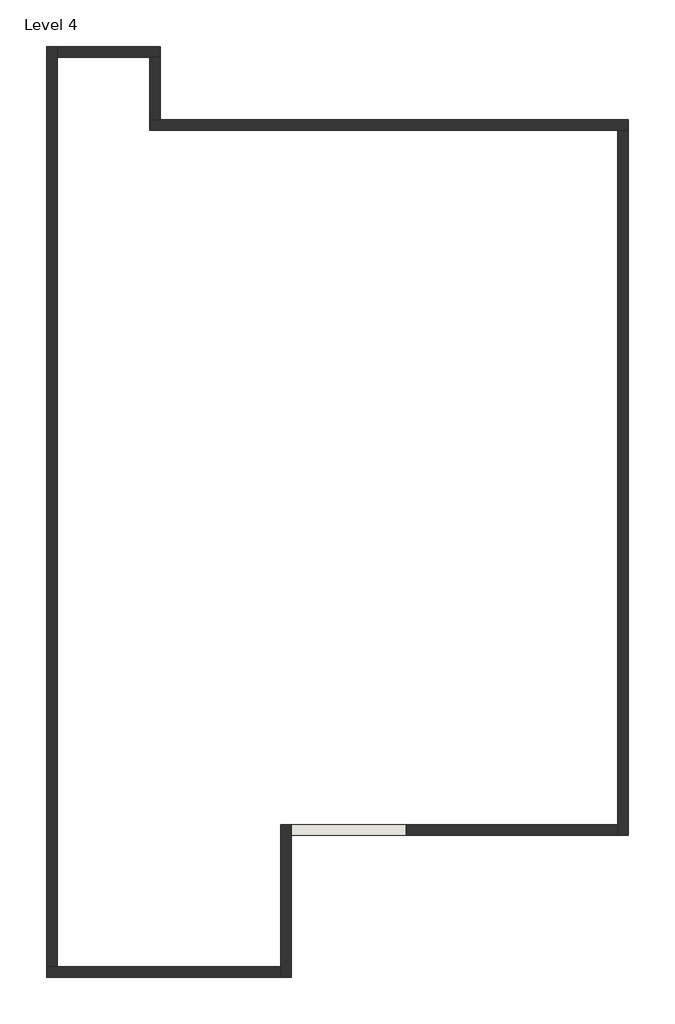
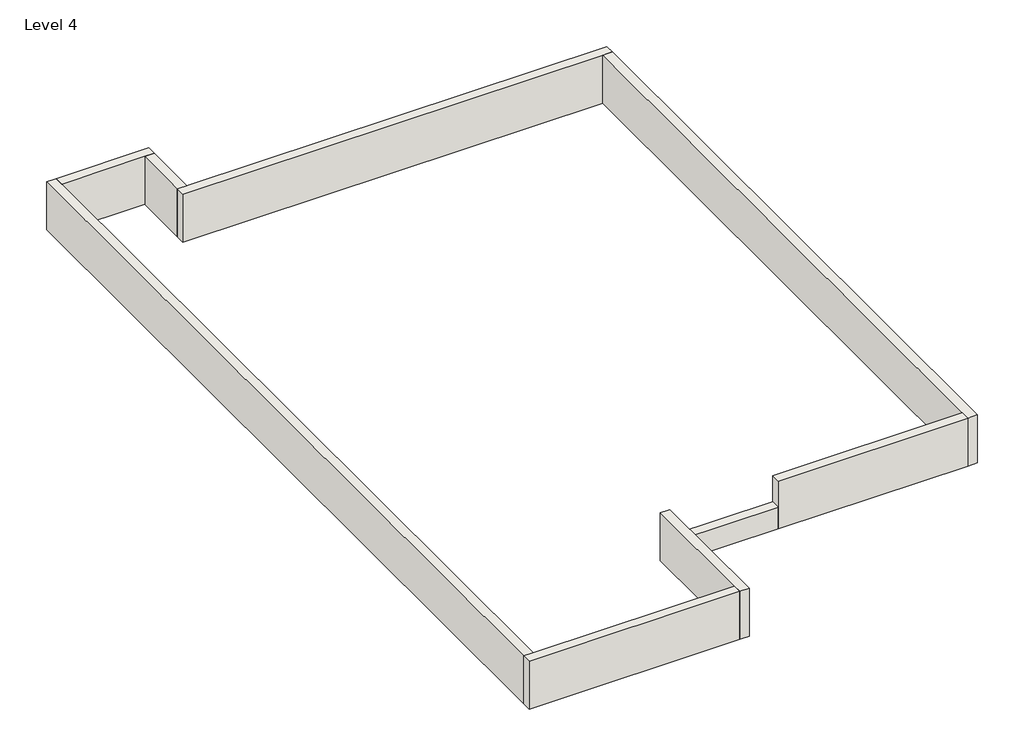
# One storey: 9 walls.
"""IFC4 building model written with IfcOpenShell, lengths in millimetres."""

from ifc_helpers import new_model, si_unit, frame, origin, place, context, project, spatial, polyline, outline, extrude, faceted_brep, element, save

model = new_model("IFC4")

# Units and contexts
model_context = context("Model", 3, world=origin())
ifc_project = project(units=[si_unit("LENGTHUNIT", "METRE", prefix="MILLI")], contexts=[model_context])

# Site, building, storey
site = spatial("IfcSite", under=ifc_project)
building = spatial("IfcBuilding", under=site)
storey = spatial("IfcBuildingStorey", under=building, Name="Level 4", Elevation=6858.0)

# Walls
placement = place(None, origin())
element("IfcWall", 1, ObjectType="9\" wall", at=placement, inside=storey, context=model_context, shape_type="Brep", body=[
    faceted_brep([(-5476.8909398, -2669.4648025, 6858.0), (-5476.8909398, -5745.6380415, 6858.0), (-5476.8909398, -5974.2380415, 6858.0), (-5476.8909398, -5974.2380415, 8077.2), (-5476.8909398, -5745.6380415, 8077.2), (-5476.8909398, -2669.4648025, 8077.2), (-5248.2909398, -2669.4648025, 6858.0), (-5248.2909398, -2669.4648025, 7414.0853363), (-5248.2909398, -2669.4648025, 8077.2), (-5248.2909398, -5974.2380415, 8077.2), (-5248.2909398, -5974.2380415, 6858.0), (-5248.2909398, -2898.0648025, 6858.0)], [[[0, 1, 2, 3, 4, 5]], [[6, 7, 8, 9, 10, 11]], [[2, 1, 0, 6, 11, 10]], [[5, 4, 3, 9, 8]], [[3, 2, 10, 9]], [[0, 5, 8, 7, 6]]]),
])
element("IfcWall", 2, ObjectType="9\" wall", at=placement, inside=storey, context=model_context, shape_type="Brep", body=[
    faceted_brep([(-5476.8909398, -5745.6380415, 6858.0), (-10315.5909398, -5745.6380415, 6858.0), (-10544.1909398, -5745.6380415, 6858.0), (-10544.1909398, -5745.6380415, 8077.2), (-10315.5909398, -5745.6380415, 8077.2), (-5476.8909398, -5745.6380415, 8077.2), (-5476.8909398, -5974.2380415, 6858.0), (-5476.8909398, -5974.2380415, 8077.2), (-10544.1909398, -5974.2380415, 8077.2), (-10544.1909398, -5974.2380415, 6858.0)], [[[0, 1, 2, 3, 4, 5]], [[6, 7, 8, 9]], [[2, 1, 0, 6, 9]], [[5, 4, 3, 8, 7]], [[0, 5, 7, 6]], [[3, 2, 9, 8]]]),
])
element("IfcWall", 3, ObjectType="9\" wall", at=placement, inside=storey, context=model_context, shape_type="Brep", body=[
    faceted_brep([(-10315.5909398, -5745.6380415, 6858.0), (-10315.5909398, 13923.3493277, 6858.0), (-10315.5909398, 14151.9493277, 6858.0), (-10315.5909398, 14151.9493277, 8077.2), (-10315.5909398, 13923.3493277, 8077.2), (-10315.5909398, -5745.6380415, 8077.2), (-10544.1909398, -5745.6380415, 6858.0), (-10544.1909398, -5745.6380415, 8077.2), (-10544.1909398, 14151.9493277, 8077.2), (-10544.1909398, 14151.9493277, 6858.0)], [[[0, 1, 2, 3, 4, 5]], [[6, 7, 8, 9]], [[2, 1, 0, 6, 9]], [[5, 4, 3, 8, 7]], [[0, 5, 7, 6]], [[3, 2, 9, 8]]]),
])
element("IfcWall", 4, ObjectType="9\" wall", at=placement, inside=storey, context=model_context, shape_type="Brep", body=[
    faceted_brep([(-8309.5689749, 12341.9351975, 6858.0), (1800.2090602, 12341.9351975, 6858.0), (2028.8090602, 12341.9351975, 6858.0), (2028.8090602, 12341.9351975, 8077.2), (1800.2090602, 12341.9351975, 8077.2), (-8309.5689749, 12341.9351975, 8077.2), (-8309.5689749, 12570.5351975, 6858.0), (-8309.5689749, 12570.5351975, 8077.2), (-8080.9689749, 12570.5351975, 8077.2), (2028.8090602, 12570.5351975, 8077.2), (2028.8090602, 12570.5351975, 6858.0), (-8080.9689749, 12570.5351975, 6858.0)], [[[0, 1, 2, 3, 4, 5]], [[6, 7, 8, 9, 10, 11]], [[2, 1, 0, 6, 11, 10]], [[5, 4, 3, 9, 8, 7]], [[3, 2, 10, 9]], [[0, 5, 7, 6]]]),
])
element("IfcWall", 5, ObjectType="9\" wall", at=placement, inside=storey, context=model_context, shape_type="Brep", body=[
    faceted_brep([(1800.2090602, 12341.9351975, 6858.0), (1800.2090602, -2669.4648025, 6858.0), (1800.2090602, -2783.7648025, 6858.0), (1800.2090602, -2898.0648025, 6858.0), (1800.2090602, -2898.0648025, 8077.2), (1800.2090602, -2669.4648025, 8077.2), (1800.2090602, 12341.9351975, 8077.2), (2028.8090602, 12341.9351975, 6858.0), (2028.8090602, 12341.9351975, 8077.2), (2028.8090602, -2898.0648025, 8077.2), (2028.8090602, -2898.0648025, 6858.0), (2028.8090602, -2783.7648025, 6858.0)], [[[0, 1, 2, 3, 4, 5, 6]], [[7, 8, 9, 10, 11]], [[3, 2, 1, 0, 7, 11, 10]], [[6, 5, 4, 9, 8]], [[0, 6, 8, 7]], [[4, 3, 10, 9]]]),
])
element("IfcWall", 6, ObjectType="9\" wall", at=placement, inside=storey, context=model_context, shape_type="Brep", body=[
    faceted_brep([(-10315.5909398, 13923.3493277, 6858.0), (-8309.5689749, 13923.3493277, 6858.0), (-8080.9689749, 13923.3493277, 6858.0), (-8080.9689749, 13923.3493277, 8077.2), (-8309.5689749, 13923.3493277, 8077.2), (-10315.5909398, 13923.3493277, 8077.2), (-10315.5909398, 14151.9493277, 6858.0), (-10315.5909398, 14151.9493277, 8077.2), (-8080.9689749, 14151.9493277, 8077.2), (-8080.9689749, 14151.9493277, 6858.0)], [[[0, 1, 2, 3, 4, 5]], [[6, 7, 8, 9]], [[2, 1, 0, 6, 9]], [[5, 4, 3, 8, 7]], [[3, 2, 9, 8]], [[0, 5, 7, 6]]]),
])
element("IfcWall", 7, ObjectType="9\" wall", at=placement, inside=storey, context=model_context, shape_type="SweptSolid", body=[
    extrude(outline(polyline([(-8309.5689749, 12570.5351975), (-8309.5689749, 13923.3493277), (-8080.9689749, 13923.3493277), (-8080.9689749, 12570.5351975), (-8309.5689749, 12570.5351975)])), frame((0.0, 0.0, 6858.0), z_axis=(0.0, 0.0, 1.0), x_axis=(1.0, 0.0, 0.0)), (0.0, 0.0, 1.0), 1219.2),
])
element("IfcWall", 8, ObjectType="9\" wall", at=placement, inside=storey, context=model_context, shape_type="Brep", body=[
    faceted_brep([(1800.2090602, -2669.4648025, 6858.0), (-2771.7909398, -2669.4648025, 6858.0), (-2771.7909398, -2669.4648025, 7414.0853363), (-2771.7909398, -2669.4648025, 8077.2), (1800.2090602, -2669.4648025, 8077.2), (1800.2090602, -2898.0648025, 6858.0), (1800.2090602, -2898.0648025, 8077.2), (-2771.7909398, -2898.0648025, 8077.2), (-2771.7909398, -2898.0648025, 7414.0853363), (-2771.7909398, -2898.0648025, 6858.0)], [[[0, 1, 2, 3, 4]], [[5, 6, 7, 8, 9]], [[1, 0, 5, 9]], [[3, 2, 1, 9, 8, 7]], [[4, 3, 7, 6]], [[0, 4, 6, 5]]]),
])
element("IfcWall", 9, ObjectType="9\" wall", at=placement, inside=storey, context=model_context, shape_type="SweptSolid", body=[
    extrude(outline(polyline([(-5248.2909398, -2669.4648025), (-2771.7909398, -2669.4648025), (-2771.7909398, -2898.0648025), (-5248.2909398, -2898.0648025), (-5248.2909398, -2669.4648025)])), frame((0.0, 0.0, 6858.0), z_axis=(0.0, 0.0, 1.0), x_axis=(1.0, 0.0, 0.0)), (0.0, 0.0, 1.0), 556.0853363),
])

save(model, "model.ifc")

# Revit data of these elements
# Type "9\" wall"
#   Assembly Code = "B2010"
#   Layers, outside or top first: 0' - 9" "Laminate, Ivory, Matte" (function 1)
# Elements 1, 2, 3, 4, 5, 6, 7, 8 (IfcWall, "9\" wall")
#   Top Offset = 0' - 0"
#   Base Offset = 0' - 0"
#   wall height = 4' - 0"
#   Phase Created = New Construction
#   Base Constraint = Level 4
#   Top Constraint = Level 5
#   Materials on its faces: "Laminate, Ivory, Matte"
# Element 9 (IfcWall, "9\" wall")
#   Top Offset = -2' - 2.10688"
#   Base Offset = 0' - 0"
#   wall height = 1' - 9.89312"
#   Phase Created = New Construction
#   Base Constraint = Level 4
#   Top Constraint = Level 5
#   Materials on its faces: "Laminate, Ivory, Matte"
# Materials
#   "Laminate, Ivory, Matte": class "Plastic", colour RGB 247 247 239, transparency 0, Description = "Plastic Laminate - Ivory, Matte", Cost = 0
